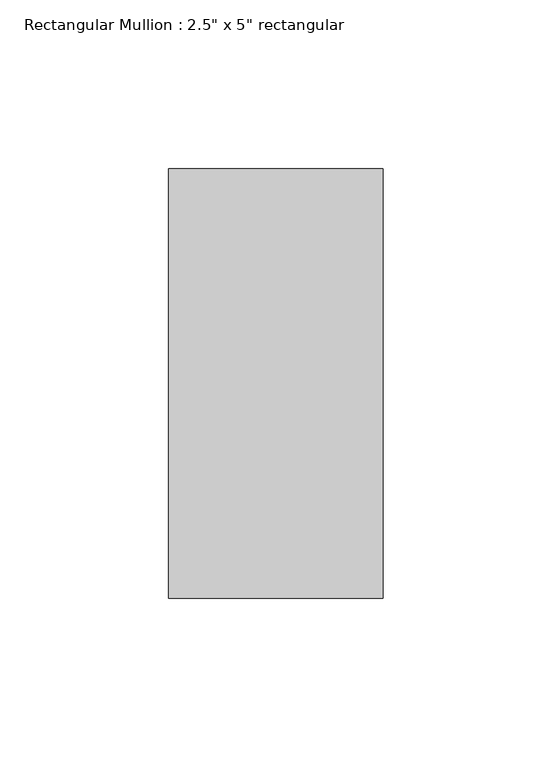
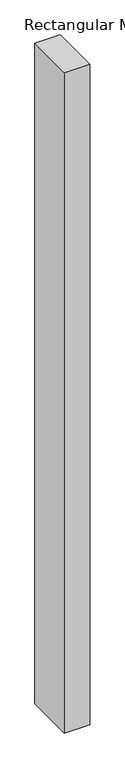
"""IFC4 building model written with IfcOpenShell, lengths in millimetres: member geometry."""

from ifc_helpers import new_model, si_unit, frame, origin, place, context, project, spatial, polyline, outline, extrude, source, transform, mapped, element, save


def member_c6b50b9a(model_context):
    return source(origin(), model_context, "Body", "SweptSolid", [
        extrude(outline(polyline([(31.75, 63.5), (31.75, -63.5), (-31.75, -63.5), (-31.75, 63.5), (31.75, 63.5)])), frame((0.0, 0.0, -1741.7653418), z_axis=(0.0, 0.0, 1.0), x_axis=(1.0, 0.0, 0.0)), (0.0, 0.0, 1.0), 1741.7653418),
    ])


if __name__ == "__main__":
    model = new_model("IFC4")
    model_context = context("Model", 3, world=origin())
    ifc_project = project(units=[si_unit("LENGTHUNIT", "METRE", prefix="MILLI")], contexts=[model_context])
    site = spatial("IfcSite", under=ifc_project)
    building = spatial("IfcBuilding", under=site)
    placement = place(None, origin())
    member_shape = member_c6b50b9a(model_context)
    element("IfcMember", 1, ObjectType="Rectangular Mullion : 2.5\" x 5\" rectangular", at=placement, inside=building, context=model_context, shape_type="MappedRepresentation", body=[
        mapped(member_shape, transform((0.0, 0.0, 0.0), x_axis=(1.0, 0.0, 0.0), y_axis=(0.0, 1.0, 0.0), z_axis=(0.0, 0.0, 1.0))),
    ])
    save(model, "model.ifc")

# Revit data of these elements
# Type "Rectangular Mullion : 2.5\" x 5\" rectangular"
#   built-in parameter 1007304 = 0.416667 (stored number, unit not read)
#   built-in parameter 1007301 = 0.104167 (stored number, unit not read)
#   built-in parameter 1007300 = 0.104167 (stored number, unit not read)
# Element 1 (IfcMember, "Rectangular Mullion : 2.5\" x 5\" rectangular")
#   Materials on its faces: "Aluminum"
# Materials
#   "Aluminum": class "Metal", colour RGB 247 247 247, transparency 0, Description = "Aluminum 6061", Cost = 0
